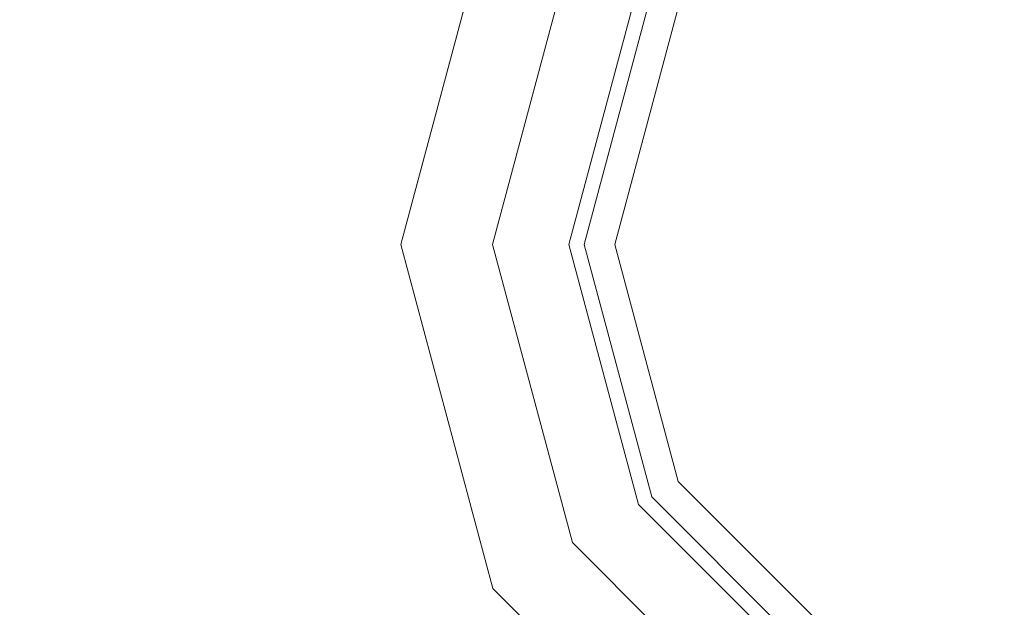
# Model space of a CAD drawing. Units: inches. Extents: x 375 to 1122, y 27 to 1069.
# Tile 137 of 155: x 731.16 to 739.094, y 892.194 to 896.928. Entities that reach past the tile are written whole.
import ezdxf

# ---------------------------------------------------------------- set-up
doc = ezdxf.new("R2010")
doc.units = ezdxf.units.IN
doc.layers.add('A-ANNO-DIMS', color=2, linetype='Continuous', lineweight=18)
doc.layers.add('Furniture', color=30, linetype='Continuous', lineweight=18)
doc.styles.get("Standard").update_dxf_attribs({"font": 'arial.ttf'})
doc.dimstyles.new('ISO-25', dxfattribs={"dimtxt": 12, "dimasz": 2.5, "dimexe": 1.5, "dimexo": 1.5, "dimtad": 1, "dimdec": 1, "dimlunit": 3, "dimtxsty": 'Standard', "dimblk": 'ARCHTICK', "dimcen": 2.5, "dimadec": 0, "dimazin": 0, "dimtfac": 1, "dimtdec": 1, "dimtmove": 0, "dimatfit": 3, "dimfxl": 1.5, "dimfxlon": 1, "dimarcsym": 0})

# ---------------------------------------------------------------- blocks, each defined once
blk = doc.blocks.new('A$C403C54AD')
at = {"linetype": 'ByBlock'}
for points, invisible_edges in [([(0.97862, 1.37069, -0.02965), (1.0802, 1.37069, -0.02965), (1.0802, 1.37069, -0.02965), (0.99223, 1.3199, -0.02965)], 5), ([(0.99223, 1.3199, -0.02965), (1.0802, 1.37069, -0.02965), (1.0802, 1.37069, -0.02965), (1.02941, 1.28271, -0.02965)], 5), ([(1.02941, 1.28271, -0.02965), (1.0802, 1.37069, -0.02965), (1.0802, 1.37069, -0.02965), (1.0802, 1.2691, -0.02965)], 5), ([(1.0802, 1.2691, -0.02965), (1.0802, 1.37069, -0.02965), (1.0802, 1.37069, -0.02965), (1.131, 1.28271, -0.02965)], 5), ([(1.16818, 1.3199, -0.02965), (1.0802, 1.37069, -0.02965), (1.0802, 1.37069, -0.02965), (1.18179, 1.37069, -0.02965)], 5), ([(1.131, 1.28271, -0.02965), (1.0802, 1.37069, -0.02965), (1.0802, 1.37069, -0.02965), (1.16818, 1.3199, -0.02965)], 5), ([(1.12792, 1.28804, -0.04658), (1.13254, 1.28005, -0.03734), (1.17085, 1.31836, -0.03734), (1.16285, 1.32297, -0.04658)], 1), ([(1.14023, 1.26672, -0.02349), (1.131, 1.28271, -0.02965), (1.16818, 1.3199, -0.02965), (1.18418, 1.31066, -0.02349)], 5), ([(1.13254, 1.28005, -0.03734), (1.14947, 1.25072, -0.02811), (1.20017, 1.30143, -0.02811), (1.17085, 1.31836, -0.03734)], 5), ([(1.14947, 1.25072, -0.02349), (1.14023, 1.26672, -0.02349), (1.18418, 1.31066, -0.02349), (1.20017, 1.30143, -0.02349)], 5), ([(1.03249, 1.28804, -0.04658), (1.02787, 1.28005, -0.03734), (1.0802, 1.26602, -0.03734), (1.0802, 1.27526, -0.04658)], 5), ([(1.0802, 1.27526, -0.04658), (1.0802, 1.26602, -0.03734), (1.13254, 1.28005, -0.03734), (1.12792, 1.28804, -0.04658)], 5), ([(1.02018, 1.26672, -0.02349), (1.02941, 1.28271, -0.02965), (1.0802, 1.2691, -0.02965), (1.0802, 1.25063, -0.02349)], 5), ([(1.0802, 1.25063, -0.02349), (1.0802, 1.2691, -0.02965), (1.131, 1.28271, -0.02965), (1.14023, 1.26672, -0.02349)], 5), ([(1.02787, 1.28005, -0.03734), (1.01094, 1.25072, -0.02811), (1.0802, 1.23216, -0.02811), (1.0802, 1.26602, -0.03734)], 5), ([(1.0802, 1.26602, -0.03734), (1.0802, 1.23216, -0.02811), (1.14947, 1.25072, -0.02811), (1.13254, 1.28005, -0.03734)], 5), ([(1.01094, 1.25072, -0.02349), (1.02018, 1.26672, -0.02349), (1.0802, 1.25063, -0.02349), (1.0802, 1.23216, -0.02349)], 5), ([(1.0802, 1.23216, -0.02349), (1.0802, 1.25063, -0.02349), (1.14023, 1.26672, -0.02349), (1.14947, 1.25072, -0.02349)], 5)]:
    blk.add_3dface(points, dxfattribs=dict(at, invisible_edges=invisible_edges))
for points in [[(1.14947, 1.25072, -0.02811), (1.14947, 1.25072, -0.02349), (1.20017, 1.30143, -0.02349), (1.20017, 1.30143, -0.02811)], [(1.01094, 1.25072, -0.02811), (1.01094, 1.25072, -0.02349), (1.0802, 1.23216, -0.02349), (1.0802, 1.23216, -0.02811)], [(1.0802, 1.23216, -0.02811), (1.0802, 1.23216, -0.02349), (1.14947, 1.25072, -0.02349), (1.14947, 1.25072, -0.02811)]]:
    blk.add_3dface(points, dxfattribs=at)
blk = doc.blocks.new('_ArchTick')
at = {"color": 0, "linetype": 'ByBlock', "const_width": 0.15}
blk.add_lwpolyline([(-0.5, -0.5), (0.5, 0.5)], dxfattribs=at)
blk = doc.blocks.new('*D88')
at = {"layer": 'A-ANNO-DIMS', "color": 0, "lineweight": -2, "transparency": 16777216}
for p, q in [((731.0073, 1052.5277), (731.0073, 1055.5277)), ((854.0073, 1052.5277), (854.0073, 1055.5277)), ((731.0073, 1054.0277), (854.0073, 1054.0277))]:
    blk.add_line(p, q, dxfattribs=at)
at = {"layer": 'Defpoints', "color": 0, "transparency": 16777216}
for p in [(854.0073, 1054.0277), (731.0073, 502.5277), (854.0073, 502.5277)]:
    blk.add_point(p, dxfattribs=at)
at = {"layer": 'A-ANNO-DIMS', "color": 0, "lineweight": -2, "transparency": 16777216, "xscale": 2.5, "yscale": 2.5, "zscale": 2.5, "rotation": 180}
blk.add_blockref('_ArchTick', (731.0073, 1054.0277), dxfattribs=at)
at = {"layer": 'A-ANNO-DIMS', "color": 0, "lineweight": -2, "transparency": 16777216, "xscale": 2.5, "yscale": 2.5, "zscale": 2.5}
blk.add_blockref('_ArchTick', (854.0073, 1054.0277), dxfattribs=at)
at = {"layer": 'A-ANNO-DIMS', "color": 0, "transparency": 16777216, "insert": (792.5073, 1060.7837), "char_height": 12, "attachment_point": 5}
blk.add_mtext('10\'-3"', dxfattribs=at)
blk = doc.blocks.new('*D91')
at = {"layer": 'A-ANNO-DIMS', "color": 0, "lineweight": -2, "transparency": 16777216}
for p, q in [((728.0073, 1052.5277), (728.0073, 1055.5277)), ((788.0073, 1052.5277), (788.0073, 1055.5277)), ((728.0073, 1054.0277), (788.0073, 1054.0277))]:
    blk.add_line(p, q, dxfattribs=at)
at = {"layer": 'Defpoints', "color": 0, "transparency": 16777216}
for p in [(788.0073, 1054.0277), (728.0073, 774.0277), (788.0073, 774.0277)]:
    blk.add_point(p, dxfattribs=at)
at = {"layer": 'A-ANNO-DIMS', "color": 0, "lineweight": -2, "transparency": 16777216, "xscale": 2.5, "yscale": 2.5, "zscale": 2.5, "rotation": 180}
blk.add_blockref('_ArchTick', (728.0073, 1054.0277), dxfattribs=at)
at = {"layer": 'A-ANNO-DIMS', "color": 0, "lineweight": -2, "transparency": 16777216, "xscale": 2.5, "yscale": 2.5, "zscale": 2.5}
blk.add_blockref('_ArchTick', (788.0073, 1054.0277), dxfattribs=at)
at = {"layer": 'A-ANNO-DIMS', "color": 0, "transparency": 16777216, "insert": (758.0073, 1060.7796), "char_height": 12, "attachment_point": 5}
blk.add_mtext('5\'-0"', dxfattribs=at)

msp = doc.modelspace()

# ---------------------------------------------------------------- block references
at = {"layer": 'Furniture', "xscale": 39.9918517141215, "yscale": 39.9918517141215, "zscale": 39.9918517141215, "rotation": 270}
msp.add_blockref('A$C403C54AD', (684.9549, 938.3156, 0.024), dxfattribs=at)

# ---------------------------------------------------------------- dimensions: what is measured, and where the dimension line sits
at = {"layer": 'A-ANNO-DIMS'}
for base, p1, p2, picture, middle in [((788.0073, 1054.0277), (728.0073, 774.0277), (788.0073, 774.0277), '*D91', (758.0073, 1060.7796)), ((854.0073, 1054.0277), (731.0073, 502.5277), (854.0073, 502.5277), '*D88', (792.5073, 1060.7837))]:
    dim = msp.add_linear_dim(base=base, p1=p1, p2=p2, dimstyle='ISO-25', override={"dimdec": 1, "dimlfac": 1, "dimrnd": 0, "dimzin": 1, "dimdsep": 46, "dimlunit": 4, "dimfrac": 2}, dxfattribs=at)
    dim.commit()
    dim.dimension.update_dxf_attribs({"geometry": picture, "text_midpoint": middle})

doc.saveas('drawing.dxf')
